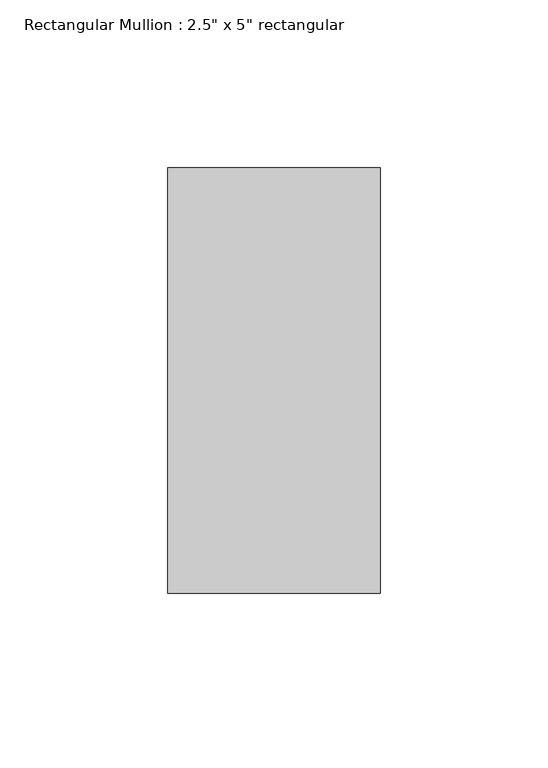
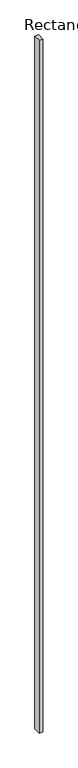
"""IFC4 building model written with IfcOpenShell, lengths in millimetres: member geometry."""

from ifc_helpers import new_model, si_unit, frame, origin, place, context, project, spatial, polyline, outline, extrude, source, transform, mapped, element, save


def member_82acb0db(model_context):
    return source(origin(), model_context, "Body", "SweptSolid", [
        extrude(outline(polyline([(0.0, 63.5), (0.0, -63.5), (-63.5, -63.5), (-63.5, 63.5), (0.0, 63.5)])), frame((0.0, 0.0, -12669.8552746), z_axis=(0.0, 0.0, 1.0), x_axis=(1.0, 0.0, 0.0)), (0.0, 0.0, 1.0), 12669.8552746),
    ])


if __name__ == "__main__":
    model = new_model("IFC4")
    model_context = context("Model", 3, world=origin())
    ifc_project = project(units=[si_unit("LENGTHUNIT", "METRE", prefix="MILLI")], contexts=[model_context])
    site = spatial("IfcSite", under=ifc_project)
    building = spatial("IfcBuilding", under=site)
    placement = place(None, origin())
    member_shape = member_82acb0db(model_context)
    element("IfcMember", 1, ObjectType="Rectangular Mullion : 2.5\" x 5\" rectangular", at=placement, inside=building, context=model_context, shape_type="MappedRepresentation", body=[
        mapped(member_shape, transform((0.0, 0.0, 0.0), x_axis=(1.0, 0.0, 0.0), y_axis=(0.0, 1.0, 0.0), z_axis=(0.0, 0.0, 1.0))),
    ])
    save(model, "model.ifc")

# Revit data of these elements
# Type "Rectangular Mullion : 2.5\" x 5\" rectangular"
#   built-in parameter 1007304 = 0.416667 (stored number, unit not read)
#   built-in parameter 1007301 = 0.104167 (stored number, unit not read)
#   built-in parameter 1007300 = 0.104167 (stored number, unit not read)
# Element 1 (IfcMember, "Rectangular Mullion : 2.5\" x 5\" rectangular")
#   Materials on its faces: "Aluminum"
# Materials
#   "Aluminum": class "Metal", colour RGB 247 247 247, transparency 0, Description = "Aluminum 6061", Cost = 0
